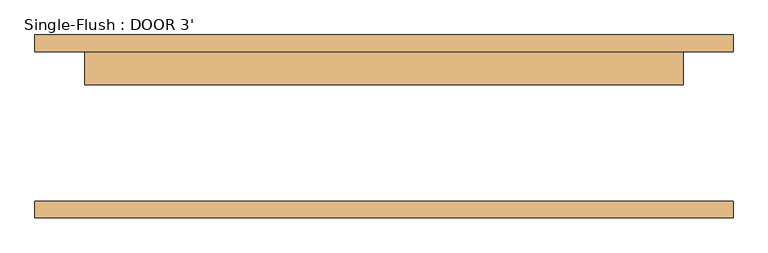
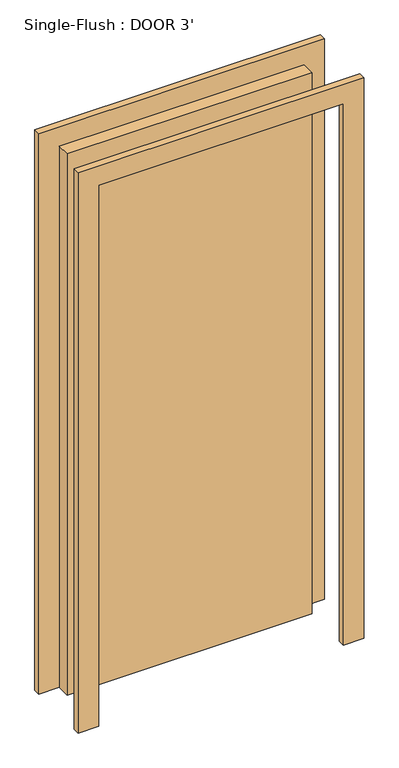
"""IFC4 building model written with IfcOpenShell, lengths in millimetres: door geometry, Single-Flush : DOOR 3'."""

from ifc_helpers import new_model, si_unit, frame, origin, origin_with_axes, place, context, project, spatial, polyline, outline, extrude, source, transform, mapped, element, save


def single_flush_door_3_0ca8825f(model_context):
    return source(origin(), model_context, "Body", "SweptSolid", [
        extrude(outline(polyline([(2209.8, -533.4), (0.0, -533.4), (0.0, -457.2), (2133.6, -457.2), (2133.6, 457.2), (0.0, 457.2), (0.0, 533.4), (2209.8, 533.4), (2209.8, -533.4)])), frame((0.0, 114.3, 0.0), z_axis=(0.0, 1.0, 0.0), x_axis=(0.0, 0.0, 1.0)), (0.0, 0.0, 1.0), 25.4),
        extrude(outline(polyline([(2209.8, 533.4), (2209.8, -533.4), (0.0, -533.4), (0.0, -457.2), (2133.6, -457.2), (2133.6, 457.2), (0.0, 457.2), (0.0, 533.4), (2209.8, 533.4)])), frame((0.0, -139.7, 0.0), z_axis=(0.0, 1.0, 0.0), x_axis=(0.0, 0.0, 1.0)), (0.0, 0.0, 1.0), 25.4),
        extrude(outline(polyline([(457.2, 63.5), (-457.2, 63.5), (-457.2, 114.3), (457.2, 114.3), (457.2, 63.5)])), origin_with_axes(), (0.0, 0.0, 1.0), 2133.6),
    ])


if __name__ == "__main__":
    model = new_model("IFC4")
    model_context = context("Model", 3, world=origin())
    ifc_project = project(units=[si_unit("LENGTHUNIT", "METRE", prefix="MILLI")], contexts=[model_context])
    site = spatial("IfcSite", under=ifc_project)
    building = spatial("IfcBuilding", under=site)
    placement = place(None, origin())
    single_flush_door_3_shape = single_flush_door_3_0ca8825f(model_context)
    element("IfcDoor", 1, ObjectType="Single-Flush : DOOR 3'", at=placement, inside=building, context=model_context, shape_type="MappedRepresentation", body=[
        mapped(single_flush_door_3_shape, transform((0.0, 0.0, 0.0), x_axis=(1.0, 0.0, 0.0), y_axis=(0.0, 1.0, 0.0), z_axis=(0.0, 0.0, 1.0))),
    ])
    save(model, "model.ifc")

# Revit data of these elements
# Type "Single-Flush : DOOR 3'"
#   Type Mark = "8"
#   Construction Type Id = "MDOOR"
#   Assembly Code = "C1020"
#   Analytic Construction = "Metal"
#   Thickness = 0' - 2"
#   Heat Transfer Coefficient (U) = 0.651978 BTU/(h·ft²·°F)
#   Height = 7' - 0"
#   Trim Projection Ext = 0' - 1"
#   Trim Projection Int = 0' - 1"
#   Trim Width = 0' - 3"
#   Width = 3' - 0"
#   Define Thermal Properties by = 1
#   Door Material = Door - Panel
#   Frame Material = Door - Frame
#   Visual Light Transmittance = 0
#   Solar Heat Gain Coefficient = 0
#   Function = (empty or 0)
#   Wall Closure = (empty or 0)
# Element 1 (IfcDoor, "Single-Flush : DOOR 3'")
#   Materials on its faces: "Door - Frame", "Door - Panel"
# Materials
#   "Door - Panel": class "Wood", colour RGB 210 159 95, transparency 0, Cost = 0
#   "Door - Frame": colour RGB 118 70 51, transparency 0, Cost = 0
